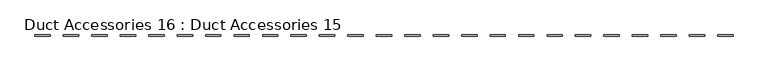
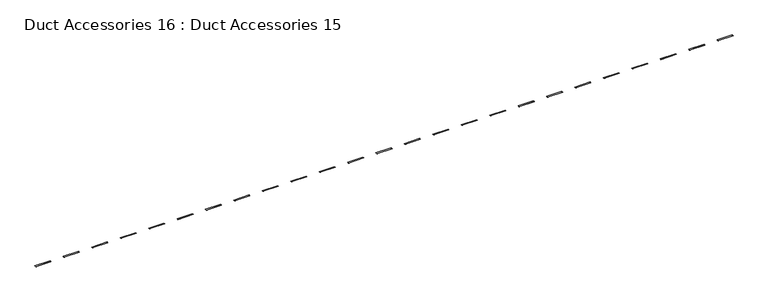
"""IFC4 building model written with IfcOpenShell, lengths in millimetres: damper geometry, Duct Accessories 16 : Duct Accessories 15."""

from ifc_helpers import new_model, si_unit, frame, origin, place, context, project, spatial, polyline, outline, extrude, source, transform, mapped, element, save


def duct_accessories_16_duct_accessories_15_820109d7(model_context):
    return source(origin(), model_context, "Body", "SweptSolid", [
        extrude(outline(polyline([(-114619.6199308, -2047.6934478), (-118734.4199308, -2047.6934478), (-118734.4199308, -1742.8934478), (-114619.6199308, -1742.8934478), (-114619.6199308, -2047.6934478)])), frame((0.0, 0.0, 14.4995117), z_axis=(0.0, 0.0, 1.0), x_axis=(1.0, 0.0, 0.0)), (0.0, 0.0, 1.0), 15.2406364),
        extrude(outline(polyline([(-106999.6199308, -2047.6934478), (-111114.4199308, -2047.6934478), (-111114.4199308, -1742.8934478), (-106999.6199308, -1742.8934478), (-106999.6199308, -2047.6934478)])), frame((0.0, 0.0, 14.4995117), z_axis=(0.0, 0.0, 1.0), x_axis=(1.0, 0.0, 0.0)), (0.0, 0.0, 1.0), 15.2406364),
        extrude(outline(polyline([(-99379.6199308, -2047.6934478), (-103494.4199308, -2047.6934478), (-103494.4199308, -1742.8934478), (-99379.6199308, -1742.8934478), (-99379.6199308, -2047.6934478)])), frame((0.0, 0.0, 14.4995117), z_axis=(0.0, 0.0, 1.0), x_axis=(1.0, 0.0, 0.0)), (0.0, 0.0, 1.0), 15.2406364),
        extrude(outline(polyline([(-91759.6199308, -2047.6934478), (-95874.4199308, -2047.6934478), (-95874.4199308, -1742.8934478), (-91759.6199308, -1742.8934478), (-91759.6199308, -2047.6934478)])), frame((0.0, 0.0, 14.4995117), z_axis=(0.0, 0.0, 1.0), x_axis=(1.0, 0.0, 0.0)), (0.0, 0.0, 1.0), 15.2406364),
        extrude(outline(polyline([(-84139.6199308, -2047.6934478), (-88254.4199308, -2047.6934478), (-88254.4199308, -1742.8934478), (-84139.6199308, -1742.8934478), (-84139.6199308, -2047.6934478)])), frame((0.0, 0.0, 14.4995117), z_axis=(0.0, 0.0, 1.0), x_axis=(1.0, 0.0, 0.0)), (0.0, 0.0, 1.0), 15.2406364),
        extrude(outline(polyline([(-76519.6199308, -2047.6934478), (-80634.4199308, -2047.6934478), (-80634.4199308, -1742.8934478), (-76519.6199308, -1742.8934478), (-76519.6199308, -2047.6934478)])), frame((0.0, 0.0, 14.4995117), z_axis=(0.0, 0.0, 1.0), x_axis=(1.0, 0.0, 0.0)), (0.0, 0.0, 1.0), 15.2406364),
        extrude(outline(polyline([(-68899.6199308, -2047.6934478), (-73014.4199308, -2047.6934478), (-73014.4199308, -1742.8934478), (-68899.6199308, -1742.8934478), (-68899.6199308, -2047.6934478)])), frame((0.0, 0.0, 14.4995117), z_axis=(0.0, 0.0, 1.0), x_axis=(1.0, 0.0, 0.0)), (0.0, 0.0, 1.0), 15.2406364),
        extrude(outline(polyline([(-61279.6199308, -2047.6934478), (-65394.4199308, -2047.6934478), (-65394.4199308, -1742.8934478), (-61279.6199308, -1742.8934478), (-61279.6199308, -2047.6934478)])), frame((0.0, 0.0, 14.4995117), z_axis=(0.0, 0.0, 1.0), x_axis=(1.0, 0.0, 0.0)), (0.0, 0.0, 1.0), 15.2406364),
        extrude(outline(polyline([(-53659.6199308, -2047.6934478), (-57774.4199308, -2047.6934478), (-57774.4199308, -1742.8934478), (-53659.6199308, -1742.8934478), (-53659.6199308, -2047.6934478)])), frame((0.0, 0.0, 14.4995117), z_axis=(0.0, 0.0, 1.0), x_axis=(1.0, 0.0, 0.0)), (0.0, 0.0, 1.0), 15.2406364),
        extrude(outline(polyline([(-46039.6199308, -2047.6934478), (-50154.4199308, -2047.6934478), (-50154.4199308, -1742.8934478), (-46039.6199308, -1742.8934478), (-46039.6199308, -2047.6934478)])), frame((0.0, 0.0, 14.4995117), z_axis=(0.0, 0.0, 1.0), x_axis=(1.0, 0.0, 0.0)), (0.0, 0.0, 1.0), 15.2406364),
        extrude(outline(polyline([(-38419.6199308, -2047.6934478), (-42534.4199308, -2047.6934478), (-42534.4199308, -1742.8934478), (-38419.6199308, -1742.8934478), (-38419.6199308, -2047.6934478)])), frame((0.0, 0.0, 14.4995117), z_axis=(0.0, 0.0, 1.0), x_axis=(1.0, 0.0, 0.0)), (0.0, 0.0, 1.0), 15.2406364),
        extrude(outline(polyline([(-30799.6199308, -2047.6934478), (-34914.4199308, -2047.6934478), (-34914.4199308, -1742.8934478), (-30799.6199308, -1742.8934478), (-30799.6199308, -2047.6934478)])), frame((0.0, 0.0, 14.4995117), z_axis=(0.0, 0.0, 1.0), x_axis=(1.0, 0.0, 0.0)), (0.0, 0.0, 1.0), 15.2406364),
        extrude(outline(polyline([(-23179.6199308, -2047.6934478), (-27294.4199308, -2047.6934478), (-27294.4199308, -1742.8934478), (-23179.6199308, -1742.8934478), (-23179.6199308, -2047.6934478)])), frame((0.0, 0.0, 14.4995117), z_axis=(0.0, 0.0, 1.0), x_axis=(1.0, 0.0, 0.0)), (0.0, 0.0, 1.0), 15.2406364),
        extrude(outline(polyline([(-15559.6199308, -2047.6934478), (-19674.4199308, -2047.6934478), (-19674.4199308, -1742.8934478), (-15559.6199308, -1742.8934478), (-15559.6199308, -2047.6934478)])), frame((0.0, 0.0, 14.4995117), z_axis=(0.0, 0.0, 1.0), x_axis=(1.0, 0.0, 0.0)), (0.0, 0.0, 1.0), 15.2406364),
        extrude(outline(polyline([(-7939.6199308, -2047.6934478), (-12054.4199308, -2047.6934478), (-12054.4199308, -1742.8934478), (-7939.6199308, -1742.8934478), (-7939.6199308, -2047.6934478)])), frame((0.0, 0.0, 14.4995117), z_axis=(0.0, 0.0, 1.0), x_axis=(1.0, 0.0, 0.0)), (0.0, 0.0, 1.0), 15.2406364),
        extrude(outline(polyline([(-319.6199308, -2047.6934478), (-4434.4199308, -2047.6934478), (-4434.4199308, -1742.8934478), (-319.6199308, -1742.8934478), (-319.6199308, -2047.6934478)])), frame((0.0, 0.0, 14.4995117), z_axis=(0.0, 0.0, 1.0), x_axis=(1.0, 0.0, 0.0)), (0.0, 0.0, 1.0), 15.2406364),
        extrude(outline(polyline([(7300.3800692, -2047.6934478), (3185.5800692, -2047.6934478), (3185.5800692, -1742.8934478), (7300.3800692, -1742.8934478), (7300.3800692, -2047.6934478)])), frame((0.0, 0.0, 14.4995117), z_axis=(0.0, 0.0, 1.0), x_axis=(1.0, 0.0, 0.0)), (0.0, 0.0, 1.0), 15.2406364),
        extrude(outline(polyline([(14920.3800692, -2047.6934478), (10805.5800692, -2047.6934478), (10805.5800692, -1742.8934478), (14920.3800692, -1742.8934478), (14920.3800692, -2047.6934478)])), frame((0.0, 0.0, 14.4995117), z_axis=(0.0, 0.0, 1.0), x_axis=(1.0, 0.0, 0.0)), (0.0, 0.0, 1.0), 15.2406364),
        extrude(outline(polyline([(22540.3800692, -2047.6934478), (18425.5800692, -2047.6934478), (18425.5800692, -1742.8934478), (22540.3800692, -1742.8934478), (22540.3800692, -2047.6934478)])), frame((0.0, 0.0, 14.4995117), z_axis=(0.0, 0.0, 1.0), x_axis=(1.0, 0.0, 0.0)), (0.0, 0.0, 1.0), 15.2406364),
        extrude(outline(polyline([(30160.3800692, -2047.6934478), (26045.5800692, -2047.6934478), (26045.5800692, -1742.8934478), (30160.3800692, -1742.8934478), (30160.3800692, -2047.6934478)])), frame((0.0, 0.0, 14.4995117), z_axis=(0.0, 0.0, 1.0), x_axis=(1.0, 0.0, 0.0)), (0.0, 0.0, 1.0), 15.2406364),
        extrude(outline(polyline([(37780.3800692, -2047.6934478), (33665.5800692, -2047.6934478), (33665.5800692, -1742.8934478), (37780.3800692, -1742.8934478), (37780.3800692, -2047.6934478)])), frame((0.0, 0.0, 14.4995117), z_axis=(0.0, 0.0, 1.0), x_axis=(1.0, 0.0, 0.0)), (0.0, 0.0, 1.0), 15.2406364),
        extrude(outline(polyline([(45400.3800692, -2047.6934478), (41285.5800692, -2047.6934478), (41285.5800692, -1742.8934478), (45400.3800692, -1742.8934478), (45400.3800692, -2047.6934478)])), frame((0.0, 0.0, 14.4995117), z_axis=(0.0, 0.0, 1.0), x_axis=(1.0, 0.0, 0.0)), (0.0, 0.0, 1.0), 15.2406364),
        extrude(outline(polyline([(53020.3800692, -2047.6934478), (48905.5800692, -2047.6934478), (48905.5800692, -1742.8934478), (53020.3800692, -1742.8934478), (53020.3800692, -2047.6934478)])), frame((0.0, 0.0, 14.4995117), z_axis=(0.0, 0.0, 1.0), x_axis=(1.0, 0.0, 0.0)), (0.0, 0.0, 1.0), 15.2406364),
        extrude(outline(polyline([(60640.3800692, -2047.6934478), (56525.5800692, -2047.6934478), (56525.5800692, -1742.8934478), (60640.3800692, -1742.8934478), (60640.3800692, -2047.6934478)])), frame((0.0, 0.0, 14.4995117), z_axis=(0.0, 0.0, 1.0), x_axis=(1.0, 0.0, 0.0)), (0.0, 0.0, 1.0), 15.2406364),
        extrude(outline(polyline([(68260.3800692, -2047.6934478), (64145.5800692, -2047.6934478), (64145.5800692, -1742.8934478), (68260.3800692, -1742.8934478), (68260.3800692, -2047.6934478)])), frame((0.0, 0.0, 14.4995117), z_axis=(0.0, 0.0, 1.0), x_axis=(1.0, 0.0, 0.0)), (0.0, 0.0, 1.0), 15.2406364),
    ])


if __name__ == "__main__":
    model = new_model("IFC4")
    model_context = context("Model", 3, world=origin())
    ifc_project = project(units=[si_unit("LENGTHUNIT", "METRE", prefix="MILLI")], contexts=[model_context])
    site = spatial("IfcSite", under=ifc_project)
    building = spatial("IfcBuilding", under=site)
    placement = place(None, origin())
    duct_accessories_16_duct_accessories_15_shape = duct_accessories_16_duct_accessories_15_820109d7(model_context)
    element("IfcDamper", 1, ObjectType="Duct Accessories 16 : Duct Accessories 15", at=placement, inside=building, context=model_context, shape_type="MappedRepresentation", body=[
        mapped(duct_accessories_16_duct_accessories_15_shape, transform((0.0, 0.0, 0.0), x_axis=(1.0, 0.0, 0.0), y_axis=(0.0, 1.0, 0.0), z_axis=(0.0, 0.0, 1.0))),
    ])
    save(model, "model.ifc")

# Revit data of these elements
# Element 1 (IfcDamper, "Duct Accessories 16 : Duct Accessories 15")
#   Materials on its faces: "Clad - White"
# Materials
#   "Clad - White": class "Wood", colour RGB 242 242 238, transparency 0, Cost = 0
